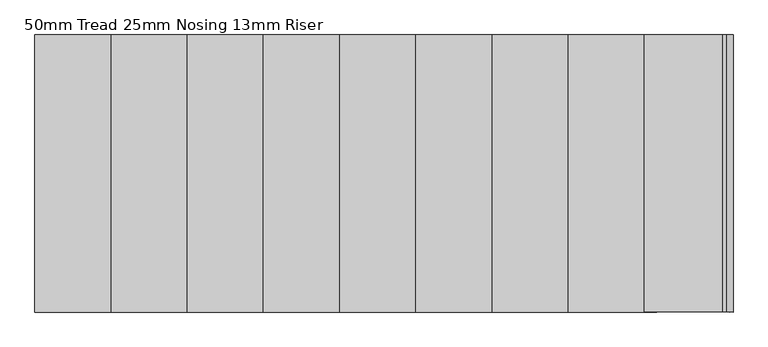
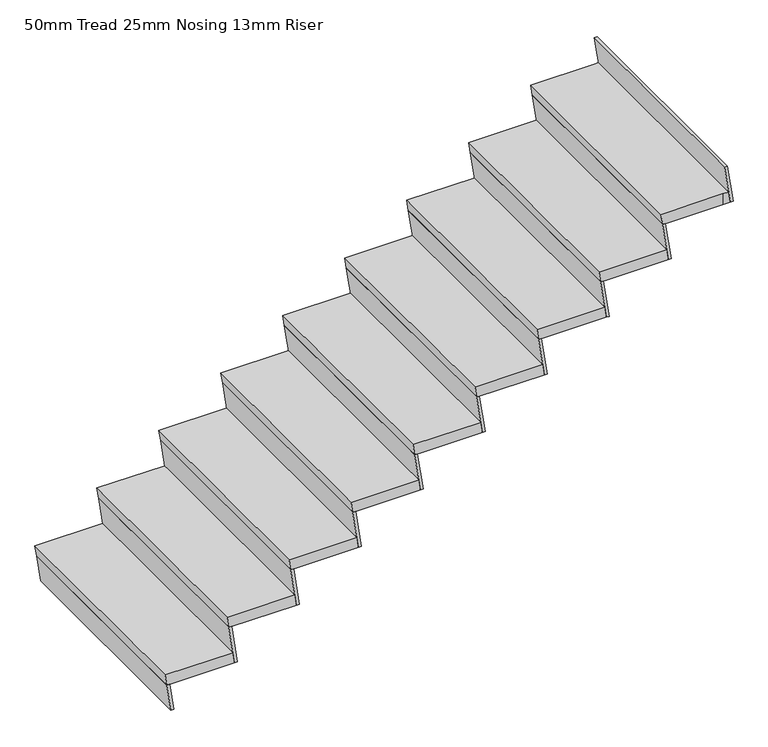
"""IFC4 building model written with IfcOpenShell, lengths in millimetres: stair flight geometry, 50mm Tread 25mm Nosing 13mm Riser."""

from ifc_helpers import new_model, si_unit, origin, place, context, project, spatial, faceted_brep, source, transform, mapped, element, save


def stair_flight_50mm_tread_25mm_nosing_13mm_riser_ecbb9275(model_context):
    return source(origin(), model_context, "Body", "Brep", [
        faceted_brep([(-99.786154, 2747.0262668, 173.9130435), (-92.598654, 2747.0262668, 123.9130435), (-92.598654, 3747.052048, 123.9130435), (-99.786154, 3747.052048, 173.9130435), (-399.786154, 3747.052048, 173.9130435), (-399.786154, 2747.0262668, 173.9130435), (-392.598654, 2747.0262668, 123.9130435), (-392.598654, 3747.052048, 123.9130435)], [[[0, 1, 2, 3]], [[3, 4, 5, 0]], [[2, 1, 6, 7]], [[4, 3, 2, 7]], [[0, 5, 6, 1]], [[5, 4, 7, 6]]]),
        faceted_brep([(-392.598654, 2747.0262668, 123.9130435), (-374.786154, 2747.0262668, 0.0), (-362.157664, 2747.0262668, 0.0), (-379.970164, 2747.0262668, 123.9130435), (-392.598654, 3747.052048, 123.9130435), (-379.970164, 3747.052048, 123.9130435), (-362.157664, 3747.052048, 0.0), (-374.786154, 3747.052048, 0.0)], [[[0, 1, 2, 3]], [[4, 5, 6, 7]], [[1, 0, 4, 7]], [[2, 1, 7, 6]], [[3, 2, 6, 5]], [[0, 3, 5, 4]]]),
        faceted_brep([(-117.598654, 2747.0262668, 297.826087), (-92.598654, 2747.0262668, 123.9130435), (-79.970164, 2747.0262668, 123.9130435), (-104.970164, 2747.0262668, 297.826087), (-117.598654, 3747.052048, 297.826087), (-104.970164, 3747.052048, 297.826087), (-79.970164, 3747.052048, 123.9130435), (-92.598654, 3747.052048, 123.9130435)], [[[0, 1, 2, 3]], [[4, 5, 6, 7]], [[1, 0, 4, 7]], [[2, 1, 7, 6]], [[3, 2, 6, 5]], [[0, 3, 5, 4]]]),
        faceted_brep([(175.213846, 3747.052048, 347.826087), (-124.786154, 3747.052048, 347.826087), (-124.786154, 2747.0262668, 347.826087), (175.213846, 2747.0262668, 347.826087), (182.401346, 3747.052048, 297.826087), (182.401346, 2747.0262668, 297.826087), (-117.598654, 2747.0262668, 297.826087), (-117.598654, 3747.052048, 297.826087)], [[[0, 1, 2, 3]], [[4, 5, 6, 7]], [[1, 0, 4, 7]], [[3, 2, 6, 5]], [[3, 5, 4, 0]], [[2, 1, 7, 6]]]),
        faceted_brep([(157.401346, 2747.0262668, 471.7391304), (182.401346, 2747.0262668, 297.826087), (195.029836, 2747.0262668, 297.826087), (170.029836, 2747.0262668, 471.7391304), (157.401346, 3747.052048, 471.7391304), (170.029836, 3747.052048, 471.7391304), (195.029836, 3747.052048, 297.826087), (182.401346, 3747.052048, 297.826087)], [[[0, 1, 2, 3]], [[4, 5, 6, 7]], [[1, 0, 4, 7]], [[2, 1, 7, 6]], [[3, 2, 6, 5]], [[0, 3, 5, 4]]]),
        faceted_brep([(450.213846, 3747.052048, 521.7391304), (150.213846, 3747.052048, 521.7391304), (150.213846, 2747.0262668, 521.7391304), (450.213846, 2747.0262668, 521.7391304), (457.401346, 3747.052048, 471.7391304), (457.401346, 2747.0262668, 471.7391304), (157.401346, 2747.0262668, 471.7391304), (157.401346, 3747.052048, 471.7391304)], [[[0, 1, 2, 3]], [[4, 5, 6, 7]], [[1, 0, 4, 7]], [[3, 2, 6, 5]], [[3, 5, 4, 0]], [[2, 1, 7, 6]]]),
        faceted_brep([(432.401346, 2747.0262668, 645.6521739), (457.401346, 2747.0262668, 471.7391304), (470.029836, 2747.0262668, 471.7391304), (445.029836, 2747.0262668, 645.6521739), (432.401346, 3747.052048, 645.6521739), (445.029836, 3747.052048, 645.6521739), (470.029836, 3747.052048, 471.7391304), (457.401346, 3747.052048, 471.7391304)], [[[0, 1, 2, 3]], [[4, 5, 6, 7]], [[1, 0, 4, 7]], [[2, 1, 7, 6]], [[3, 2, 6, 5]], [[0, 3, 5, 4]]]),
        faceted_brep([(725.213846, 3747.052048, 695.6521739), (425.213846, 3747.052048, 695.6521739), (425.213846, 2747.0262668, 695.6521739), (725.213846, 2747.0262668, 695.6521739), (732.401346, 3747.052048, 645.6521739), (732.401346, 2747.0262668, 645.6521739), (432.401346, 2747.0262668, 645.6521739), (432.401346, 3747.052048, 645.6521739)], [[[0, 1, 2, 3]], [[4, 5, 6, 7]], [[1, 0, 4, 7]], [[3, 2, 6, 5]], [[3, 5, 4, 0]], [[2, 1, 7, 6]]]),
        faceted_brep([(707.401346, 2747.0262668, 819.5652174), (732.401346, 2747.0262668, 645.6521739), (745.029836, 2747.0262668, 645.6521739), (720.029836, 2747.0262668, 819.5652174), (707.401346, 3747.052048, 819.5652174), (720.029836, 3747.052048, 819.5652174), (745.029836, 3747.052048, 645.6521739), (732.401346, 3747.052048, 645.6521739)], [[[0, 1, 2, 3]], [[4, 5, 6, 7]], [[1, 0, 4, 7]], [[2, 1, 7, 6]], [[3, 2, 6, 5]], [[0, 3, 5, 4]]]),
        faceted_brep([(1000.213846, 3747.052048, 869.5652174), (700.213846, 3747.052048, 869.5652174), (700.213846, 2747.0262668, 869.5652174), (1000.213846, 2747.0262668, 869.5652174), (1007.401346, 3747.052048, 819.5652174), (1007.401346, 2747.0262668, 819.5652174), (707.401346, 2747.0262668, 819.5652174), (707.401346, 3747.052048, 819.5652174)], [[[0, 1, 2, 3]], [[4, 5, 6, 7]], [[1, 0, 4, 7]], [[3, 2, 6, 5]], [[3, 5, 4, 0]], [[2, 1, 7, 6]]]),
        faceted_brep([(982.401346, 2747.0262668, 993.4782609), (1007.401346, 2747.0262668, 819.5652174), (1020.029836, 2747.0262668, 819.5652174), (995.029836, 2747.0262668, 993.4782609), (982.401346, 3747.052048, 993.4782609), (995.029836, 3747.052048, 993.4782609), (1020.029836, 3747.052048, 819.5652174), (1007.401346, 3747.052048, 819.5652174)], [[[0, 1, 2, 3]], [[4, 5, 6, 7]], [[1, 0, 4, 7]], [[2, 1, 7, 6]], [[3, 2, 6, 5]], [[0, 3, 5, 4]]]),
        faceted_brep([(1275.213846, 3747.052048, 1043.4782609), (975.213846, 3747.052048, 1043.4782609), (975.213846, 2747.0262668, 1043.4782609), (1275.213846, 2747.0262668, 1043.4782609), (1282.401346, 3747.052048, 993.4782609), (1282.401346, 2747.0262668, 993.4782609), (982.401346, 2747.0262668, 993.4782609), (982.401346, 3747.052048, 993.4782609)], [[[0, 1, 2, 3]], [[4, 5, 6, 7]], [[1, 0, 4, 7]], [[3, 2, 6, 5]], [[3, 5, 4, 0]], [[2, 1, 7, 6]]]),
        faceted_brep([(1257.401346, 2747.0262668, 1167.3913043), (1282.401346, 2747.0262668, 993.4782609), (1295.029836, 2747.0262668, 993.4782609), (1270.029836, 2747.0262668, 1167.3913043), (1257.401346, 3747.052048, 1167.3913043), (1270.029836, 3747.052048, 1167.3913043), (1295.029836, 3747.052048, 993.4782609), (1282.401346, 3747.052048, 993.4782609)], [[[0, 1, 2, 3]], [[4, 5, 6, 7]], [[1, 0, 4, 7]], [[2, 1, 7, 6]], [[3, 2, 6, 5]], [[0, 3, 5, 4]]]),
        faceted_brep([(1550.213846, 3747.052048, 1217.3913043), (1250.213846, 3747.052048, 1217.3913043), (1250.213846, 2747.0262668, 1217.3913043), (1550.213846, 2747.0262668, 1217.3913043), (1557.401346, 3747.052048, 1167.3913043), (1557.401346, 2747.0262668, 1167.3913043), (1257.401346, 2747.0262668, 1167.3913043), (1257.401346, 3747.052048, 1167.3913043)], [[[0, 1, 2, 3]], [[4, 5, 6, 7]], [[1, 0, 4, 7]], [[3, 2, 6, 5]], [[3, 5, 4, 0]], [[2, 1, 7, 6]]]),
        faceted_brep([(1532.401346, 2747.0262668, 1341.3043478), (1557.401346, 2747.0262668, 1167.3913043), (1570.029836, 2747.0262668, 1167.3913043), (1545.029836, 2747.0262668, 1341.3043478), (1532.401346, 3747.052048, 1341.3043478), (1545.029836, 3747.052048, 1341.3043478), (1570.029836, 3747.052048, 1167.3913043), (1557.401346, 3747.052048, 1167.3913043)], [[[0, 1, 2, 3]], [[4, 5, 6, 7]], [[1, 0, 4, 7]], [[2, 1, 7, 6]], [[3, 2, 6, 5]], [[0, 3, 5, 4]]]),
        faceted_brep([(1825.213846, 3747.052048, 1391.3043478), (1525.213846, 3747.052048, 1391.3043478), (1525.213846, 2747.0262668, 1391.3043478), (1825.213846, 2747.0262668, 1391.3043478), (1832.401346, 3747.052048, 1341.3043478), (1832.401346, 2747.0262668, 1341.3043478), (1532.401346, 2747.0262668, 1341.3043478), (1532.401346, 3747.052048, 1341.3043478)], [[[0, 1, 2, 3]], [[4, 5, 6, 7]], [[1, 0, 4, 7]], [[3, 2, 6, 5]], [[3, 5, 4, 0]], [[2, 1, 7, 6]]]),
        faceted_brep([(2082.401346, 2747.0262668, 1689.1304348), (2107.401346, 2747.0262668, 1515.2173913), (2120.029836, 2747.0262668, 1515.2173913), (2095.029836, 2747.0262668, 1689.1304348), (2082.401346, 3747.052048, 1689.1304348), (2095.029836, 3747.052048, 1689.1304348), (2120.029836, 3747.052048, 1515.2173913), (2107.401346, 3747.052048, 1515.2173913)], [[[0, 1, 2, 3]], [[4, 5, 6, 7]], [[1, 0, 4, 7]], [[2, 1, 7, 6]], [[3, 2, 6, 5]], [[0, 3, 5, 4]]]),
        faceted_brep([(1807.401346, 2747.0262668, 1515.2173913), (1832.401346, 2747.0262668, 1341.3043478), (1845.029836, 2747.0262668, 1341.3043478), (1820.029836, 2747.0262668, 1515.2173913), (1807.401346, 3747.052048, 1515.2173913), (1820.029836, 3747.052048, 1515.2173913), (1845.029836, 3747.052048, 1341.3043478), (1832.401346, 3747.052048, 1341.3043478)], [[[0, 1, 2, 3]], [[4, 5, 6, 7]], [[1, 0, 4, 7]], [[2, 1, 7, 6]], [[3, 2, 6, 5]], [[0, 3, 5, 4]]]),
        faceted_brep([(2100.213846, 3747.052048, 1565.2173913), (2075.213846, 3747.052048, 1565.2173913), (1800.213846, 3747.052048, 1565.2173913), (1800.213846, 2747.0262668, 1565.2173913), (2075.213846, 2747.0262668, 1565.2173913), (2100.213846, 2747.0262668, 1565.2173913), (2107.401346, 3747.052048, 1515.2173913), (2107.401346, 2747.0262668, 1515.2173913), (2075.213846, 2747.0262668, 1515.2173913), (1807.401346, 2747.0262668, 1515.2173913), (1807.401346, 3747.052048, 1515.2173913), (2075.213846, 3747.052048, 1515.2173913)], [[[0, 1, 2, 3, 4, 5]], [[6, 7, 8, 9, 10, 11]], [[1, 0, 6, 11]], [[4, 3, 9, 8]], [[5, 4, 8, 7]], [[5, 7, 6, 0]], [[3, 2, 10, 9]], [[2, 1, 11, 10]]]),
    ])


if __name__ == "__main__":
    model = new_model("IFC4")
    model_context = context("Model", 3, world=origin())
    ifc_project = project(units=[si_unit("LENGTHUNIT", "METRE", prefix="MILLI")], contexts=[model_context])
    site = spatial("IfcSite", under=ifc_project)
    building = spatial("IfcBuilding", under=site)
    placement = place(None, origin())
    stair_flight_50mm_tread_25mm_nosing_13mm_riser_shape = stair_flight_50mm_tread_25mm_nosing_13mm_riser_ecbb9275(model_context)
    element("IfcStairFlight", 1, ObjectType="50mm Tread 25mm Nosing 13mm Riser", at=placement, inside=building, context=model_context, shape_type="MappedRepresentation", body=[
        mapped(stair_flight_50mm_tread_25mm_nosing_13mm_riser_shape, transform((0.0, 0.0, 0.0), x_axis=(1.0, 0.0, 0.0), y_axis=(0.0, 1.0, 0.0), z_axis=(0.0, 0.0, 1.0))),
    ])
    save(model, "model.ifc")
